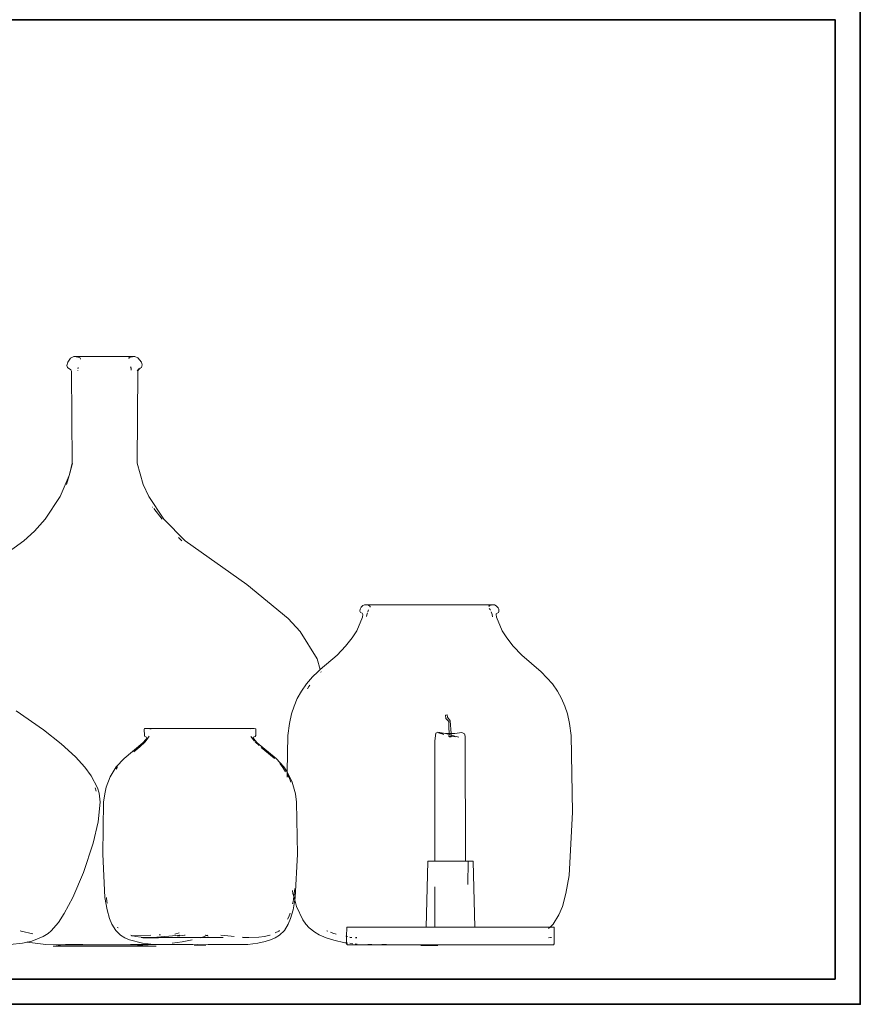
# Model space of a CAD drawing. Units: millimetres. Extents: x 446512 to 447461, y 70395 to 70610.
# Tile 8 of 39: x 446729.93 to 446746.57, y 70453.38 to 70472.88. Entities that reach past the tile are written whole.
import ezdxf

# ---------------------------------------------------------------- set-up
doc = ezdxf.new("R2010")
doc.units = ezdxf.units.MM
doc.layers.add('A-FURN', color=7, linetype='Continuous', lineweight=35)
doc.layers.add('A-FURN-DECO', color=8, linetype='Continuous', lineweight=13)

msp = doc.modelspace()

# ---------------------------------------------------------------- linework, layer by layer
at = {"layer": 'A-FURN'}
for p in [(446746.5728, 70473.3815), (446686.5728, 70453.3815)]:
    msp.add_line(p, (446746.5728, 70453.3815), dxfattribs=at)
for points in [[(446699.4288, 70473.3815), (446746.5728, 70473.3815), (446746.5728, 70453.3815), (446699.4288, 70453.3815)], [(446699.9288, 70472.8815), (446746.0728, 70472.8815), (446746.0728, 70453.8815), (446699.9288, 70453.8815)]]:
    msp.add_lwpolyline(points, close=True, dxfattribs=at)
at = {"layer": 'A-FURN-DECO'}
for p, q in [((446730.8833, 70466.1012), (446730.9391, 70466.1776)), ((446731.0042, 70466.2085), (446730.9391, 70466.1776)), ((446731.0042, 70466.2085), (446731.0132, 70466.2085)), ((446731.0132, 70466.2085), (446731.1207, 70466.1917)), ((446731.0132, 70466.2085), (446731.2691, 70466.2085)), ((446731.1207, 70466.1917), (446731.1347, 70466.1656)), ((446731.3461, 70466.2079), (446731.2691, 70466.2085)), ((446731.4113, 70466.2085), (446731.3461, 70466.2079)), ((446731.658, 70466.2079), (446731.4113, 70466.2085)), ((446731.7262, 70466.2085), (446731.658, 70466.2079)), ((446732.2118, 70466.2085), (446731.7262, 70466.2085)), ((446732.1271, 70466.2047), (446732.0841, 70466.1969)), ((446732.0841, 70466.1969), (446732.1181, 70466.2)), ((446732.1075, 70466.1944), (446732.0902, 70466.1656)), ((446732.1181, 70466.2), (446732.1075, 70466.1944)), ((446732.1181, 70466.2), (446732.2118, 70466.2085)), ((446732.1271, 70466.2047), (446732.1181, 70466.2)), ((446732.2736, 70466.1857), (446732.2118, 70466.2085)), ((446732.3417, 70466.1012), (446732.2736, 70466.1857)), ((446730.8833, 70466.1012), (446730.8682, 70466.0336)), ((446730.8811, 70465.9946), (446730.8682, 70466.0336)), ((446730.8811, 70465.9946), (446730.947, 70465.9496)), ((446731.0915, 70465.9946), (446731.0864, 70465.9802)), ((446731.1347, 70466.1656), (446731.1345, 70466.1603)), ((446732.0902, 70466.1656), (446732.0904, 70466.162)), ((446732.1237, 70466.0051), (446732.1311, 70465.9802)), ((446732.1386, 70465.9802), (446732.1299, 70466.0044)), ((446732.3271, 70465.9893), (446732.2935, 70465.9653)), ((446732.3139, 70465.9771), (446732.3439, 70465.9946)), ((446732.3139, 70465.9771), (446732.3271, 70465.9893)), ((446732.3562, 70466.0483), (446732.3417, 70466.1012)), ((446732.3439, 70465.9946), (446732.3562, 70466.0483)), ((446730.9569, 70465.9223), (446730.947, 70465.9496)), ((446730.9694, 70464.0979), (446730.9569, 70465.9223)), ((446731.0848, 70465.933), (446731.0846, 70465.9262)), ((446731.0864, 70465.9802), (446731.086, 70465.9694)), ((446732.1398, 70465.9425), (446732.1386, 70465.9802)), ((446732.2684, 70465.9262), (446732.2556, 70464.0979)), ((446732.2935, 70465.9653), (446732.2585, 70465.9262)), ((446732.2585, 70465.9262), (446732.2826, 70465.9484)), ((446732.2684, 70465.9262), (446732.2826, 70465.9484)), ((446732.2826, 70465.9484), (446732.3139, 70465.9771)), ((446732.2826, 70465.9484), (446732.2935, 70465.9653)), ((446732.2935, 70465.9653), (446732.3139, 70465.9771)), ((446730.9237, 70463.9024), (446730.9694, 70464.0979)), ((446730.979, 70464.0979), (446730.9237, 70463.9024)), ((446732.2556, 70464.0979), (446732.3788, 70463.6734)), ((446730.7358, 70463.4377), (446730.9105, 70463.856)), ((446730.9105, 70463.856), (446730.8588, 70463.6734)), ((446730.9237, 70463.9024), (446730.9105, 70463.856)), ((446732.4891, 70463.4377), (446732.3788, 70463.6734)), ((446730.4374, 70462.9881), (446730.7358, 70463.4377)), ((446732.7876, 70462.9881), (446732.4891, 70463.4377)), ((446732.5646, 70463.2268), (446732.5637, 70463.228)), ((446732.7509, 70462.9881), (446732.5851, 70463.2005)), ((446730.2237, 70462.7516), (446730.4374, 70462.9881)), ((446733.2078, 70462.5633), (446732.7876, 70462.9881)), ((446730.0171, 70462.5633), (446730.2237, 70462.7516)), ((446728.7945, 70461.6966), (446730.0171, 70462.5633)), ((446733.1423, 70462.5633), (446733.0753, 70462.6275)), ((446734.4305, 70461.6966), (446733.2078, 70462.5633)), ((446735.2469, 70461.0217), (446734.4305, 70461.6966)), ((446736.6675, 70461.1665), (446736.672, 70461.2043)), ((446736.6675, 70461.1665), (446736.6778, 70461.1443)), ((446736.672, 70461.2043), (446736.6928, 70461.2467)), ((446736.7104, 70461.1262), (446736.6778, 70461.1443)), ((446736.6928, 70461.2467), (446736.724, 70461.2766)), ((446736.7269, 70461.1029), (446736.7104, 70461.1262)), ((446736.724, 70461.2766), (446736.7601, 70461.2922)), ((446736.7601, 70461.2922), (446736.8402, 70461.2859)), ((446736.7601, 70461.2922), (446737.7066, 70461.2922)), ((446736.8162, 70461.1319), (446736.8049, 70461.0975)), ((446736.8356, 70461.1907), (446736.8233, 70461.1532)), ((446736.8402, 70461.2859), (446736.8698, 70461.2616)), ((446736.8698, 70461.2616), (446736.8721, 70461.2477)), ((446737.7166, 70461.2917), (446737.7066, 70461.2922)), ((446737.7166, 70461.2917), (446739.2834, 70461.2922)), ((446739.2148, 70461.2876), (446739.2654, 70461.2894)), ((446739.2334, 70461.2785), (446739.2194, 70461.2624)), ((446739.2276, 70461.2189), (446739.2475, 70461.2038)), ((446739.2654, 70461.2894), (446739.2334, 70461.2785)), ((446739.2475, 70461.2038), (446739.2523, 70461.1901)), ((446739.264, 70461.1568), (446739.2665, 70461.1497)), ((446739.2834, 70461.2922), (446739.2654, 70461.2894)), ((446739.2703, 70461.1387), (446739.2843, 70461.099)), ((446739.2862, 70461.2922), (446739.2834, 70461.2922)), ((446739.2862, 70461.2922), (446739.3308, 70461.2917)), ((446739.3675, 70461.2749), (446739.3308, 70461.2917)), ((446739.3617, 70461.1029), (446739.3676, 70461.1155)), ((446739.4042, 70461.2332), (446739.3675, 70461.2749)), ((446739.3676, 70461.1155), (446739.4088, 70461.1426)), ((446739.4166, 70461.2043), (446739.4042, 70461.2332)), ((446739.4088, 70461.1426), (446739.42, 70461.1607)), ((446739.42, 70461.1607), (446739.4166, 70461.2043)), ((446735.4828, 70460.7655), (446735.2469, 70461.0217)), ((446736.6032, 70460.7809), (446736.7182, 70461.0462)), ((446736.7182, 70461.0462), (446736.7269, 70461.1029)), ((446736.8049, 70461.0975), (446736.798, 70461.0595)), ((446739.2843, 70461.099), (446739.2912, 70461.0585)), ((446739.3704, 70461.0462), (446739.3617, 70461.1029)), ((446739.4854, 70460.7809), (446739.3704, 70461.0462)), ((446735.4828, 70460.7655), (446735.8235, 70460.2208)), ((446736.512, 70460.6397), (446736.6032, 70460.7809)), ((446739.5766, 70460.6397), (446739.4854, 70460.7809)), ((446736.3845, 70460.4776), (446736.512, 70460.6397)), ((446739.7041, 70460.4776), (446739.5766, 70460.6397)), ((446736.2148, 70460.2981), (446736.3845, 70460.4776)), ((446739.8739, 70460.2981), (446739.7041, 70460.4776)), ((446735.8835, 70460.0107), (446735.8235, 70460.2208)), ((446735.8835, 70460.0107), (446736.2148, 70460.2981)), ((446740.2527, 70459.9694), (446739.8739, 70460.2981)), ((446735.7302, 70459.8661), (446735.8359, 70459.9694)), ((446735.8359, 70459.9694), (446735.8835, 70460.0107)), ((446735.8978, 70459.9607), (446735.8953, 70459.9694)), ((446740.4795, 70459.7258), (446740.2527, 70459.9694)), ((446735.6092, 70459.7258), (446735.7302, 70459.8661)), ((446735.5091, 70459.5825), (446735.428, 70459.4364)), ((446735.6092, 70459.7258), (446735.5091, 70459.5825)), ((446735.6566, 70459.6736), (446735.6287, 70459.6282)), ((446735.6786, 70459.7023), (446735.6566, 70459.6736)), ((446740.5795, 70459.5825), (446740.4795, 70459.7258)), ((446740.6606, 70459.4364), (446740.5795, 70459.5825)), ((446735.364, 70459.2875), (446735.428, 70459.4364)), ((446740.7246, 70459.2875), (446740.6606, 70459.4364)), ((446730.4065, 70458.8154), (446729.8611, 70459.1958)), ((446735.3151, 70459.136), (446735.364, 70459.2875)), ((446740.7735, 70459.136), (446740.7246, 70459.2875)), ((446735.2722, 70458.943), (446735.3151, 70459.136)), ((446738.3952, 70459.1121), (446738.3619, 70459.1103)), ((446738.3702, 70459.0448), (446738.3619, 70459.1103)), ((446738.4262, 70458.9829), (446738.3702, 70459.0448)), ((446738.4028, 70459.067), (446738.3952, 70459.1121)), ((446738.4552, 70458.997), (446738.4028, 70459.067)), ((446738.4286, 70458.8707), (446738.4262, 70458.9829)), ((446738.4552, 70458.997), (446738.4724, 70458.742)), ((446740.8164, 70458.943), (446740.7735, 70459.136)), ((446730.7523, 70458.543), (446730.4065, 70458.8154)), ((446732.4033, 70458.841), (446732.3986, 70458.831)), ((446732.4007, 70458.7021), (446732.3986, 70458.831)), ((446732.4148, 70458.8463), (446732.4033, 70458.841)), ((446732.4507, 70458.8463), (446732.4148, 70458.8463)), ((446732.4148, 70458.8463), (446732.5054, 70458.8398)), ((446732.4585, 70458.8469), (446732.4507, 70458.8463)), ((446732.4585, 70458.8469), (446732.5751, 70458.8469)), ((446732.5054, 70458.8398), (446732.5111, 70458.8364)), ((446732.5054, 70458.8398), (446732.5357, 70458.837)), ((446732.5357, 70458.837), (446732.5372, 70458.8371)), ((446732.7302, 70458.8463), (446732.5751, 70458.8469)), ((446732.7302, 70458.8463), (446732.9623, 70458.8463)), ((446732.9623, 70458.8463), (446733.2204, 70458.8469)), ((446733.2246, 70458.8469), (446733.2204, 70458.8469)), ((446733.2246, 70458.8469), (446733.2286, 70458.8469)), ((446733.2286, 70458.8469), (446733.4979, 70458.8463)), ((446733.7878, 70458.8463), (446733.4979, 70458.8463)), ((446734.035, 70458.8469), (446733.7878, 70458.8463)), ((446734.0468, 70458.8469), (446734.035, 70458.8469)), ((446734.0468, 70458.8469), (446734.264, 70458.8469)), ((446734.4417, 70458.8463), (446734.264, 70458.8469)), ((446734.5514, 70458.8463), (446734.4417, 70458.8463)), ((446734.4926, 70458.8365), (446734.5514, 70458.8463)), ((446734.5537, 70458.8463), (446734.5514, 70458.8463)), ((446734.5537, 70458.8463), (446734.5752, 70458.8469)), ((446734.5752, 70458.8469), (446734.6038, 70458.8374)), ((446734.6038, 70458.8374), (446734.6037, 70458.7021)), ((446735.2424, 70458.7064), (446735.2722, 70458.943)), ((446738.2099, 70458.7697), (446738.1689, 70458.7506)), ((446738.3586, 70458.7422), (446738.2099, 70458.7697)), ((446738.432, 70458.7421), (446738.4286, 70458.8707)), ((446740.8462, 70458.7064), (446740.8164, 70458.943)), ((446732.3107, 70458.4825), (446732.4128, 70458.5807)), ((446732.4349, 70458.6333), (446732.3691, 70458.5617)), ((446732.4007, 70458.7021), (446732.4087, 70458.688)), ((446732.4087, 70458.688), (446732.4441, 70458.6744)), ((446732.4714, 70458.6494), (446732.4128, 70458.5807)), ((446732.4484, 70458.6592), (446732.4349, 70458.6333)), ((446732.4441, 70458.6744), (446732.4484, 70458.6592)), ((446732.4714, 70458.6494), (446732.497, 70458.6946)), ((446734.5802, 70458.5953), (446734.508, 70458.6874)), ((446734.5588, 70458.6729), (446734.5555, 70458.6649)), ((446734.5555, 70458.6649), (446734.5628, 70458.6436)), ((446734.5942, 70458.6867), (446734.5588, 70458.6729)), ((446734.5628, 70458.6436), (446734.6353, 70458.5617)), ((446734.6037, 70458.7021), (446734.5942, 70458.6867)), ((446734.6708, 70458.5046), (446734.5959, 70458.5765)), ((446735.2289, 70457.9838), (446735.2424, 70458.7064)), ((446738.152, 70458.6011), (446738.1689, 70458.7506)), ((446738.152, 70456.2151), (446738.152, 70458.6011)), ((446738.3289, 70458.7265), (446738.2237, 70458.7595)), ((446738.2237, 70458.7595), (446738.3586, 70458.7422)), ((446738.3586, 70458.7422), (446738.432, 70458.7421)), ((446738.4325, 70458.7225), (446738.3586, 70458.7422)), ((446738.4333, 70458.6938), (446738.4128, 70458.7002)), ((446738.4325, 70458.7225), (446738.432, 70458.7421)), ((446738.432, 70458.7421), (446738.4724, 70458.742)), ((446738.4744, 70458.7118), (446738.4325, 70458.7225)), ((446738.4327, 70458.716), (446738.4326, 70458.7198)), ((446738.4333, 70458.6938), (446738.433, 70458.7068)), ((446738.454, 70458.6873), (446738.4333, 70458.6938)), ((446738.4337, 70458.6791), (446738.4333, 70458.6938)), ((446738.4603, 70458.6777), (446738.4337, 70458.6791)), ((446738.454, 70458.6873), (446738.4762, 70458.6854)), ((446738.4603, 70458.6777), (446738.4767, 70458.6773)), ((446738.4724, 70458.742), (446738.4744, 70458.7118)), ((446738.4724, 70458.742), (446738.5494, 70458.7419)), ((446738.6265, 70458.6728), (446738.4744, 70458.7118)), ((446738.4747, 70458.7064), (446738.4756, 70458.6929)), ((446738.4762, 70458.6854), (446738.4767, 70458.6773)), ((446738.4762, 70458.6854), (446738.5539, 70458.6789)), ((446738.5494, 70458.7419), (446738.6843, 70458.7623)), ((446738.6843, 70458.7623), (446738.739, 70458.7414)), ((446738.7517, 70458.6927), (446738.739, 70458.7414)), ((446738.7517, 70458.6927), (446738.7544, 70456.2151)), ((446740.8738, 70457.1884), (446740.8462, 70458.7064)), ((446731.0357, 70458.2815), (446730.7523, 70458.543)), ((446732.3691, 70458.5617), (446731.9981, 70458.2474)), ((446732.1883, 70458.3832), (446732.3107, 70458.4825)), ((446734.6353, 70458.5617), (446735.0063, 70458.2474)), ((446734.9715, 70458.2571), (446734.7097, 70458.4695)), ((446731.2193, 70458.0782), (446731.0357, 70458.2815)), ((446731.9981, 70458.2474), (446731.8436, 70458.0814)), ((446734.9814, 70458.2474), (446734.9715, 70458.2571)), ((446735.0063, 70458.2474), (446735.1608, 70458.0814)), ((446731.346, 70457.9066), (446731.2193, 70458.0782)), ((446731.8436, 70458.0814), (446731.7203, 70457.8843)), ((446731.8404, 70458.0402), (446731.8607, 70458.07)), ((446731.8607, 70458.07), (446731.8702, 70458.0814)), ((446735.1437, 70458.07), (446735.0787, 70458.1481)), ((446735.1965, 70457.9838), (446735.1437, 70458.07)), ((446735.1608, 70458.0814), (446735.2289, 70457.9838)), ((446731.346, 70457.9066), (446731.472, 70457.6668)), ((446731.7203, 70457.8843), (446731.6434, 70457.6797)), ((446735.227, 70457.934), (446735.2289, 70457.9838)), ((446735.2283, 70457.9319), (446735.227, 70457.934)), ((446735.2273, 70457.8789), (446735.2283, 70457.9319)), ((446735.266, 70457.8703), (446735.2283, 70457.9319)), ((446735.2289, 70457.9838), (446735.3277, 70457.7829)), ((446735.2985, 70457.7829), (446735.266, 70457.8703)), ((446731.4258, 70457.6668), (446731.4452, 70457.6057)), ((446731.5045, 70457.5652), (446731.472, 70457.6668)), ((446731.6434, 70457.6797), (446731.6142, 70457.5483)), ((446735.3277, 70457.7829), (446735.3902, 70457.5483)), ((446731.5264, 70457.3867), (446731.5045, 70457.5652)), ((446731.6142, 70457.5483), (446731.5938, 70457.3872)), ((446735.3902, 70457.5483), (446735.4106, 70457.3872)), ((446731.5264, 70457.3867), (446731.486, 70456.9946)), ((446731.5938, 70457.3872), (446731.5751, 70456.3533)), ((446735.4106, 70457.3872), (446735.4293, 70456.3533)), ((446740.8102, 70455.9322), (446740.8738, 70457.1884)), ((446731.486, 70456.9946), (446731.3876, 70456.5742)), ((446731.3876, 70456.5742), (446731.1964, 70455.9925)), ((446731.5751, 70456.3533), (446731.6184, 70455.4977)), ((446735.4293, 70456.3533), (446735.386, 70455.4977)), ((446737.9805, 70454.9097), (446738.0104, 70456.2106)), ((446738.0104, 70456.2106), (446738.0158, 70456.2151)), ((446738.0158, 70456.2151), (446738.0545, 70456.2151)), ((446738.0545, 70456.2151), (446738.0567, 70456.2151)), ((446738.0567, 70456.2151), (446738.0741, 70456.2151)), ((446738.0741, 70456.2151), (446738.078, 70456.2151)), ((446738.078, 70456.2151), (446738.0797, 70456.2151)), ((446738.0797, 70456.2151), (446738.0915, 70456.2151)), ((446738.0915, 70456.2151), (446738.0976, 70456.2151)), ((446738.0976, 70456.2151), (446738.1012, 70456.2151)), ((446738.1012, 70456.2151), (446738.1032, 70456.2152)), ((446738.1032, 70456.2152), (446738.1059, 70456.2151)), ((446738.1059, 70456.2151), (446738.1103, 70456.2152)), ((446738.1134, 70456.2152), (446738.1103, 70456.2152)), ((446738.1103, 70456.2152), (446738.1104, 70456.2106)), ((446738.1134, 70456.2152), (446738.1153, 70456.2152)), ((446738.1153, 70456.2152), (446738.1207, 70456.2152)), ((446738.1298, 70456.2152), (446738.1207, 70456.2152)), ((446738.1321, 70456.2151), (446738.1298, 70456.2152)), ((446738.1321, 70456.2151), (446738.1404, 70456.2151)), ((446738.1404, 70456.2151), (446738.1428, 70456.2152)), ((446738.1428, 70456.2152), (446738.1442, 70456.2152)), ((446738.1442, 70456.2152), (446738.152, 70456.2151)), ((446738.152, 70456.2106), (446738.152, 70456.2151)), ((446738.1632, 70456.2151), (446738.152, 70456.2151)), ((446738.1632, 70456.2151), (446738.1773, 70456.2152)), ((446738.2261, 70456.2152), (446738.1773, 70456.2152)), ((446738.2335, 70456.2151), (446738.2261, 70456.2152)), ((446738.2335, 70456.2151), (446738.2722, 70456.2151)), ((446738.2722, 70456.2151), (446738.2815, 70456.2152)), ((446738.2815, 70456.2152), (446738.3437, 70456.2152)), ((446738.3545, 70456.2151), (446738.3437, 70456.2152)), ((446738.3545, 70456.2151), (446738.3766, 70456.2152)), ((446738.4409, 70456.2151), (446738.3766, 70456.2152)), ((446738.4409, 70456.2151), (446738.4446, 70456.2152)), ((446738.4446, 70456.2152), (446738.5132, 70456.2152)), ((446738.528, 70456.2151), (446738.5132, 70456.2152)), ((446738.528, 70456.2151), (446738.5708, 70456.2151)), ((446738.5708, 70456.2151), (446738.5797, 70456.2152)), ((446738.6046, 70456.2151), (446738.5797, 70456.2152)), ((446738.6077, 70456.2151), (446738.6046, 70456.2151)), ((446738.6114, 70456.2152), (446738.6077, 70456.2151)), ((446738.6114, 70456.2152), (446738.6141, 70456.2151)), ((446738.6141, 70456.2151), (446738.6159, 70456.2151)), ((446738.6159, 70456.2151), (446738.6388, 70456.2152)), ((446738.6481, 70456.2151), (446738.6388, 70456.2152)), ((446738.6664, 70456.2151), (446738.6481, 70456.2151)), ((446738.6664, 70456.2151), (446738.6701, 70456.2152)), ((446738.6701, 70456.2152), (446738.7208, 70456.2152)), ((446738.7273, 70456.2151), (446738.7208, 70456.2152)), ((446738.7273, 70456.2151), (446738.7457, 70456.2151)), ((446738.7505, 70456.2151), (446738.7457, 70456.2151)), ((446738.7544, 70456.2151), (446738.7505, 70456.2151)), ((446738.7557, 70456.2151), (446738.7544, 70456.2151)), ((446738.7544, 70456.2151), (446738.7544, 70456.2106)), ((446738.7598, 70456.2152), (446738.7557, 70456.2151)), ((446738.7614, 70456.2152), (446738.7598, 70456.2152)), ((446738.7614, 70456.2152), (446738.7715, 70456.2151)), ((446738.7747, 70456.2151), (446738.7715, 70456.2151)), ((446738.7882, 70456.2151), (446738.7747, 70456.2151)), ((446738.7916, 70456.2151), (446738.7882, 70456.2151)), ((446738.7916, 70456.2151), (446738.8003, 70456.2152)), ((446738.8101, 70456.2152), (446738.8003, 70456.2152)), ((446738.8101, 70456.2152), (446738.8033, 70455.7542)), ((446738.8131, 70456.2152), (446738.8101, 70456.2152)), ((446738.8161, 70456.2151), (446738.8131, 70456.2152)), ((446738.8161, 70456.2151), (446738.8348, 70456.2151)), ((446738.8348, 70456.2151), (446738.8389, 70456.2151)), ((446738.8389, 70456.2151), (446738.8432, 70456.2151)), ((446738.8432, 70456.2151), (446738.8587, 70456.2151)), ((446738.8587, 70456.2151), (446738.8614, 70456.2151)), ((446738.8614, 70456.2151), (446738.8635, 70456.2151)), ((446738.8635, 70456.2151), (446738.8704, 70456.2151)), ((446738.8704, 70456.2151), (446738.9048, 70456.2151)), ((446738.9099, 70456.2106), (446738.9048, 70456.2151)), ((446738.9398, 70454.9097), (446738.9099, 70456.2106)), ((446730.9856, 70455.4981), (446731.1964, 70455.9925)), ((446740.7468, 70455.5735), (446740.8102, 70455.9322)), ((446735.3586, 70455.5141), (446735.3818, 70455.6745)), ((446738.152, 70454.9097), (446738.152, 70455.7067)), ((446730.9856, 70455.4981), (446730.8144, 70455.1775)), ((446731.6184, 70455.4977), (446731.6616, 70455.2534)), ((446731.6603, 70455.414), (446731.6482, 70455.4977)), ((446735.3418, 70455.5735), (446735.3304, 70455.6377)), ((446735.3586, 70455.5141), (446735.3418, 70455.5735)), ((446735.3441, 70455.414), (446735.3586, 70455.5141)), ((446735.3772, 70455.4481), (446735.3586, 70455.5141)), ((446735.386, 70455.4977), (446735.3772, 70455.4481)), ((446740.6748, 70455.3187), (446740.7468, 70455.5735)), ((446731.6689, 70455.383), (446731.6603, 70455.414)), ((446735.3336, 70455.3701), (446735.3441, 70455.414)), ((446735.3772, 70455.4481), (446735.3428, 70455.2534)), ((446735.4138, 70455.3187), (446735.3772, 70455.4481)), ((446735.5349, 70455.055), (446735.4138, 70455.3187)), ((446740.6066, 70455.1522), (446740.6748, 70455.3187)), ((446730.6985, 70455.0013), (446730.8144, 70455.1775)), ((446731.6616, 70455.2534), (446731.7106, 70455.0799)), ((446731.7106, 70455.0799), (446731.757, 70454.9665)), ((446735.236, 70455.066), (446735.2602, 70455.1126)), ((446735.2938, 70455.0799), (446735.2474, 70454.9665)), ((446735.2602, 70455.1126), (446735.2863, 70455.1895)), ((446735.3428, 70455.2534), (446735.2938, 70455.0799)), ((446740.4945, 70454.97), (446740.6066, 70455.1522)), ((446730.5557, 70454.8359), (446730.6985, 70455.0013)), ((446731.757, 70454.9665), (446731.8334, 70454.8423)), ((446731.8785, 70454.8931), (446731.8649, 70454.9058)), ((446735.2474, 70454.9665), (446735.171, 70454.8423)), ((446735.5941, 70454.97), (446735.5349, 70455.055)), ((446735.66, 70454.8984), (446735.5941, 70454.97)), ((446735.773, 70454.8101), (446735.66, 70454.8984)), ((446736.4047, 70454.7243), (446736.405, 70454.9097)), ((446737.9805, 70454.9097), (446736.405, 70454.9097)), ((446738.152, 70454.9097), (446737.9805, 70454.9097)), ((446738.152, 70454.9097), (446738.9398, 70454.9097)), ((446740.4028, 70454.9097), (446738.9398, 70454.9097)), ((446740.4028, 70454.9097), (446740.4306, 70454.9096)), ((446740.4028, 70454.8829), (446740.4306, 70454.9096)), ((446740.4306, 70454.9096), (446740.4945, 70454.97)), ((446740.4394, 70454.9096), (446740.4306, 70454.9096)), ((446740.4508, 70454.9097), (446740.4394, 70454.9096)), ((446740.4508, 70454.9097), (446740.5153, 70454.9097)), ((446740.5158, 70454.5773), (446740.5153, 70454.9097)), ((446729.9624, 70454.8305), (446729.9417, 70454.8359)), ((446729.9624, 70454.8305), (446730.1914, 70454.7795)), ((446730.3982, 70454.724), (446730.1704, 70454.6337)), ((446730.3982, 70454.724), (446730.4968, 70454.7867)), ((446730.5557, 70454.8359), (446730.4968, 70454.7867)), ((446731.8334, 70454.8423), (446731.9283, 70454.7522)), ((446731.9283, 70454.7522), (446732.013, 70454.6995)), ((446732.013, 70454.6995), (446732.1079, 70454.6569)), ((446732.1755, 70454.7386), (446732.1313, 70454.7507)), ((446732.1471, 70454.7375), (446732.1755, 70454.7386)), ((446732.1755, 70454.7386), (446732.5295, 70454.7522)), ((446732.2261, 70454.7248), (446732.1755, 70454.7386)), ((446732.3373, 70454.7107), (446732.2261, 70454.7248)), ((446732.5049, 70454.6999), (446732.3339, 70454.7056)), ((446732.5686, 70454.7053), (446732.3373, 70454.7107)), ((446732.3668, 70454.6999), (446732.5049, 70454.6999)), ((446732.6822, 70454.6999), (446732.5049, 70454.6999)), ((446732.8853, 70454.729), (446732.5686, 70454.7053)), ((446732.5686, 70454.7053), (446733.5352, 70454.7053)), ((446732.6928, 70454.7585), (446732.7165, 70454.7594)), ((446732.8853, 70454.729), (446732.8868, 70454.729)), ((446733.0934, 70454.7522), (446732.8868, 70454.729)), ((446733.0026, 70454.7729), (446733.0893, 70454.7938)), ((446733.1977, 70454.7522), (446733.0533, 70454.729)), ((446733.1003, 70454.753), (446733.098, 70454.7527)), ((446733.1977, 70454.7522), (446733.2054, 70454.7522)), ((446733.5352, 70454.7053), (446733.5204, 70454.6995)), ((446733.6306, 70454.7431), (446733.5352, 70454.7053)), ((446733.96, 70454.7053), (446733.5352, 70454.7053)), ((446733.6306, 70454.7431), (446733.6089, 70454.7522)), ((446733.6166, 70454.7522), (446733.6306, 70454.7431)), ((446733.6306, 70454.7431), (446733.6332, 70454.7442)), ((446733.6535, 70454.7522), (446733.6332, 70454.7442)), ((446733.6332, 70454.7442), (446733.6644, 70454.729)), ((446733.9139, 70454.7522), (446734.1176, 70454.729)), ((446734.1176, 70454.729), (446734.181, 70454.7247)), ((446734.3329, 70454.7145), (446734.4698, 70454.7053)), ((446734.4698, 70454.7053), (446734.3582, 70454.7053)), ((446734.4698, 70454.7053), (446734.6671, 70454.7107)), ((446734.6671, 70454.7107), (446734.7783, 70454.7248)), ((446734.7783, 70454.7248), (446734.8821, 70454.7486)), ((446734.8821, 70454.7486), (446734.8898, 70454.7522)), ((446734.9914, 70454.6995), (446734.8965, 70454.6569)), ((446734.9871, 70454.7975), (446735.0604, 70454.8316)), ((446735.0761, 70454.7522), (446734.9914, 70454.6995)), ((446735.0604, 70454.8316), (446735.0737, 70454.8423)), ((446735.171, 70454.8423), (446735.0761, 70454.7522)), ((446735.8577, 70454.7602), (446735.773, 70454.8101)), ((446735.9971, 70454.6977), (446735.8577, 70454.7602)), ((446736.1492, 70454.6487), (446735.9971, 70454.6977)), ((446736.0149, 70454.8377), (446736.0353, 70454.8295)), ((446736.088, 70454.8083), (446736.13, 70454.7914)), ((446736.13, 70454.7914), (446736.1961, 70454.7724)), ((446736.3858, 70454.7279), (446736.4047, 70454.7243)), ((446736.4045, 70454.5973), (446736.4047, 70454.7243)), ((446736.4047, 70454.7243), (446736.4187, 70454.7217)), ((446736.4692, 70454.7121), (446736.4993, 70454.7063)), ((446736.4692, 70454.7016), (446736.4787, 70454.7016)), ((446736.4787, 70454.7016), (446736.507, 70454.7014)), ((446736.4993, 70454.7063), (446736.5061, 70454.7061)), ((446736.5785, 70454.7035), (446736.6084, 70454.7024)), ((446736.5791, 70454.7009), (446736.6084, 70454.7007)), ((446740.4416, 70454.7016), (446740.4031, 70454.7013)), ((446740.46, 70454.7016), (446740.4416, 70454.7016)), ((446729.9853, 70454.5956), (446729.746, 70454.5677)), ((446730.0822, 70454.6155), (446729.9853, 70454.5956)), ((446730.0749, 70454.6165), (446730.0822, 70454.6155)), ((446730.1704, 70454.6337), (446730.0822, 70454.6155)), ((446730.0822, 70454.6155), (446730.4504, 70454.566)), ((446731.179, 70454.5609), (446730.4504, 70454.566)), ((446730.592, 70454.5318), (446730.61, 70454.5318)), ((446730.61, 70454.5318), (446730.7427, 70454.5502)), ((446730.61, 70454.5318), (446732.5814, 70454.5318)), ((446731.179, 70454.5609), (446730.7427, 70454.5502)), ((446730.9717, 70454.566), (446730.8395, 70454.566)), ((446731.05, 70454.5641), (446730.9717, 70454.566)), ((446731.05, 70454.5641), (446731.179, 70454.5609)), ((446731.1825, 70454.5636), (446731.05, 70454.5641)), ((446731.179, 70454.5609), (446731.4366, 70454.5619)), ((446731.4366, 70454.5619), (446731.1825, 70454.5636)), ((446731.4366, 70454.5619), (446731.4537, 70454.5618)), ((446731.4537, 70454.5618), (446731.5666, 70454.5624)), ((446731.5666, 70454.5624), (446731.5835, 70454.5609)), ((446731.6069, 70454.5623), (446731.5835, 70454.5609)), ((446731.6268, 70454.5626), (446731.6069, 70454.5623)), ((446731.6429, 70454.5626), (446731.6268, 70454.5626)), ((446731.6518, 70454.5627), (446731.6429, 70454.5626)), ((446731.6669, 70454.5625), (446731.6518, 70454.5627)), ((446731.6913, 70454.5625), (446731.6669, 70454.5625)), ((446731.7481, 70454.5618), (446731.6913, 70454.5625)), ((446731.7481, 70454.5618), (446731.7917, 70454.5621)), ((446732.1231, 70454.564), (446731.7917, 70454.5621)), ((446732.0386, 70454.5609), (446731.7917, 70454.5621)), ((446732.0386, 70454.5609), (446732.1231, 70454.564)), ((446732.0386, 70454.5609), (446732.2669, 70454.5502)), ((446732.1079, 70454.6569), (446732.3602, 70454.5915)), ((446732.483, 70454.566), (446732.1231, 70454.564)), ((446732.2669, 70454.5502), (446732.5814, 70454.5318)), ((446732.3602, 70454.5915), (446732.5892, 70454.568)), ((446732.483, 70454.566), (446732.5844, 70454.566)), ((446732.633, 70454.5318), (446732.5814, 70454.5318)), ((446732.5892, 70454.568), (446732.5844, 70454.566)), ((446732.5892, 70454.568), (446732.6865, 70454.568)), ((446732.6865, 70454.568), (446732.7529, 70454.566)), ((446732.7664, 70454.5678), (446732.7529, 70454.566)), ((446732.7664, 70454.5678), (446733.3597, 70454.5656)), ((446733.1502, 70454.6165), (446732.953, 70454.5915)), ((446733.3463, 70454.6569), (446733.1502, 70454.6165)), ((446733.3597, 70454.5656), (446733.458, 70454.5606)), ((446733.3853, 70454.5521), (446733.4006, 70454.5521)), ((446733.458, 70454.5606), (446733.4006, 70454.5521)), ((446733.4006, 70454.5521), (446733.6191, 70454.5521)), ((446733.4898, 70454.5614), (446733.458, 70454.5606)), ((446733.4614, 70454.5656), (446733.4898, 70454.5614)), ((446733.4898, 70454.5614), (446733.4956, 70454.5615)), ((446733.4956, 70454.5615), (446733.5031, 70454.5606)), ((446733.5031, 70454.5606), (446733.5108, 70454.5609)), ((446733.5108, 70454.5609), (446733.5132, 70454.5606)), ((446733.6659, 70454.5656), (446733.5132, 70454.5606)), ((446733.5132, 70454.5606), (446733.6191, 70454.5521)), ((446734.4132, 70454.568), (446733.6659, 70454.5656)), ((446734.4132, 70454.568), (446734.4463, 70454.568)), ((446734.6442, 70454.5915), (446734.4463, 70454.568)), ((446734.6442, 70454.5915), (446734.7929, 70454.6235)), ((446734.8965, 70454.6569), (446734.7929, 70454.6235)), ((446736.3676, 70454.6017), (446736.1492, 70454.6487)), ((446736.4045, 70454.5973), (446736.3676, 70454.6017)), ((446736.4045, 70454.5773), (446736.4045, 70454.5973)), ((446736.4279, 70454.5945), (446736.4045, 70454.5973)), ((446736.4202, 70454.5585), (446736.4045, 70454.5773)), ((446736.9353, 70454.5585), (446736.4202, 70454.5585)), ((446736.5293, 70454.5825), (446736.469, 70454.5896)), ((446736.6117, 70454.5727), (446736.5727, 70454.5773)), ((446736.8257, 70454.5667), (446736.8409, 70454.5672)), ((446736.8467, 70454.5672), (446736.8409, 70454.5672)), ((446736.8961, 70454.567), (446736.8467, 70454.5672)), ((446736.9002, 70454.5665), (446736.8961, 70454.567)), ((446736.9517, 70454.5596), (446736.9353, 70454.5585)), ((446736.9596, 70454.5585), (446736.9517, 70454.5596)), ((446736.9596, 70454.5585), (446737.2294, 70454.5585)), ((446737.1931, 70454.5659), (446737.0983, 70454.5663)), ((446737.2294, 70454.5585), (446737.1019, 70454.5597)), ((446737.1964, 70454.5656), (446737.1931, 70454.5659)), ((446737.2434, 70454.5602), (446737.2294, 70454.5585)), ((446737.2586, 70454.5585), (446737.2434, 70454.5602)), ((446737.2586, 70454.5585), (446737.989, 70454.5585)), ((446737.8727, 70454.5438), (446737.9956, 70454.5564)), ((446737.8727, 70454.5438), (446738.2098, 70454.5438)), ((446737.9956, 70454.5564), (446737.989, 70454.5585)), ((446737.9956, 70454.5564), (446738.029, 70454.5585)), ((446738.0631, 70454.5564), (446738.029, 70454.5585)), ((446738.0766, 70454.5585), (446738.0631, 70454.5564)), ((446738.0766, 70454.5585), (446738.1118, 70454.5564)), ((446738.1118, 70454.5564), (446738.1267, 70454.5585)), ((446738.2098, 70454.5438), (446738.1118, 70454.5564)), ((446738.1267, 70454.5585), (446739.985, 70454.5585)), ((446739.985, 70454.5585), (446740.1112, 70454.5593)), ((446740.2019, 70454.5585), (446740.1112, 70454.5593)), ((446740.2019, 70454.5585), (446740.218, 70454.559)), ((446740.218, 70454.559), (446740.2194, 70454.5588)), ((446740.218, 70454.559), (446740.2209, 70454.559)), ((446740.2209, 70454.559), (446740.2979, 70454.5585)), ((446740.2979, 70454.5585), (446740.3122, 70454.5588)), ((446740.3122, 70454.5588), (446740.3136, 70454.5588)), ((446740.3136, 70454.5588), (446740.3762, 70454.5585)), ((446740.3762, 70454.5585), (446740.4191, 70454.5586)), ((446740.4191, 70454.5586), (446740.4361, 70454.5585)), ((446740.445, 70454.5586), (446740.4361, 70454.5585)), ((446740.5001, 70454.5585), (446740.445, 70454.5586)), ((446740.5001, 70454.5585), (446740.5158, 70454.5773))]:
    msp.add_line(p, q, dxfattribs=at)

doc.saveas('drawing.dxf')
